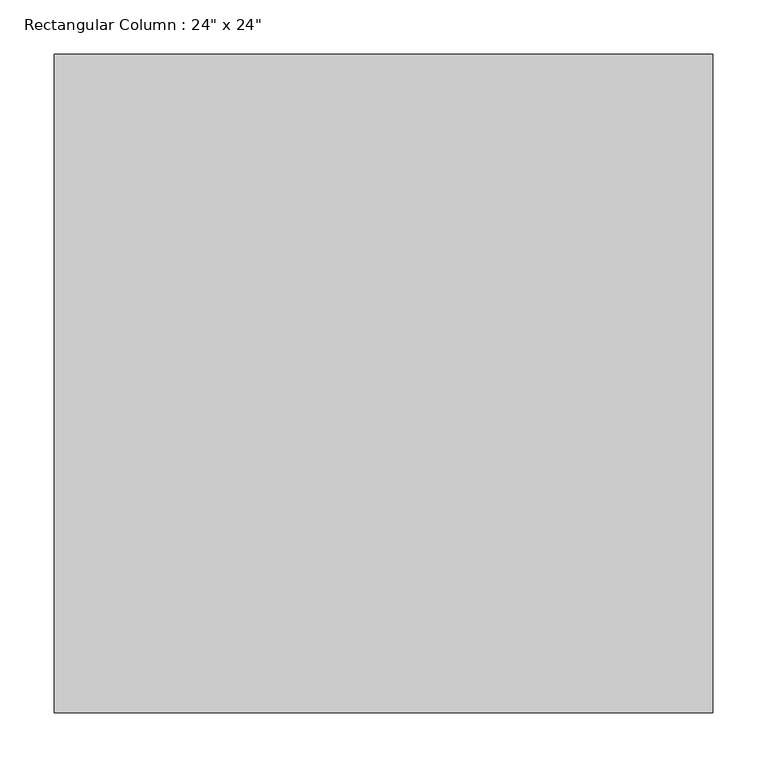
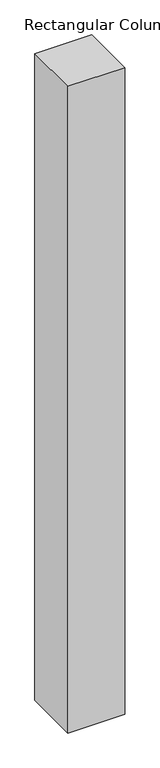
"""IFC4 building model written with IfcOpenShell, lengths in millimetres: column geometry."""

from ifc_helpers import new_model, si_unit, frame, origin, place, context, project, spatial, polyline, outline, extrude, source, transform, mapped, element, save


def column_feb29232(model_context):
    return source(origin(), model_context, "Body", "SweptSolid", [
        extrude(outline(polyline([(304.8, 304.8), (304.8, -304.8), (-304.8, -304.8), (-304.8, 304.8), (304.8, 304.8)])), frame((0.0, 0.0, 3657.6), z_axis=(0.0, 0.0, 1.0), x_axis=(1.0, 0.0, 0.0)), (0.0, 0.0, 1.0), 7315.2),
    ])


if __name__ == "__main__":
    model = new_model("IFC4")
    model_context = context("Model", 3, world=origin())
    ifc_project = project(units=[si_unit("LENGTHUNIT", "METRE", prefix="MILLI")], contexts=[model_context])
    site = spatial("IfcSite", under=ifc_project)
    building = spatial("IfcBuilding", under=site)
    placement = place(None, origin())
    column_shape = column_feb29232(model_context)
    element("IfcColumn", 1, ObjectType="Rectangular Column : 24\" x 24\"", at=placement, inside=building, context=model_context, shape_type="MappedRepresentation", body=[
        mapped(column_shape, transform((0.0, 0.0, 0.0), x_axis=(1.0, 0.0, 0.0), y_axis=(0.0, 1.0, 0.0), z_axis=(0.0, 0.0, 1.0))),
    ])
    save(model, "model.ifc")

# Revit data of these elements
# Type "Rectangular Column : 24\" x 24\""
#   Assembly Code = "B1010200"
#   Depth = 2' - 0"
#   Offset Base = 0' - 0"
#   Offset Top = 0' - 0"
#   Width = 2' - 0"
#   Material = none
